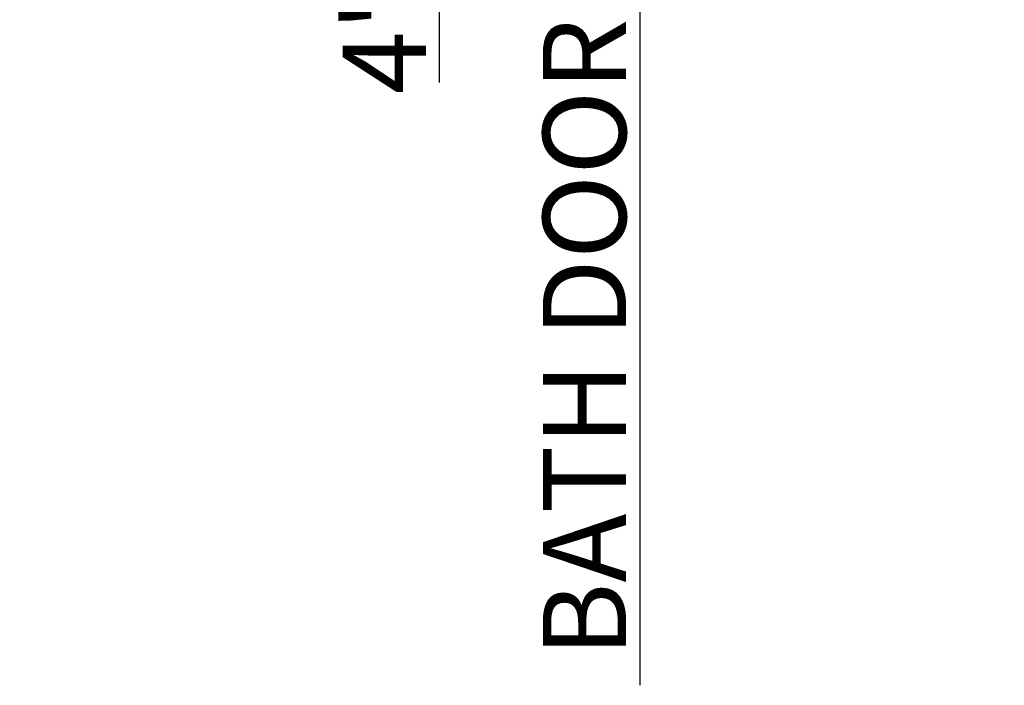
# Model space of a CAD drawing. Units: inches. Extents: x 1102 to 2414, y 295 to 1561.
# Tile 2 of 11: x 1539 to 1965, y 295 to 583. Entities that reach past the tile are written whole.
import ezdxf

# ---------------------------------------------------------------- set-up
doc = ezdxf.new("R2010")
doc.units = ezdxf.units.IN
doc.layers.add('A-ANNO-DIMS', color=2, linetype='Continuous', lineweight=18)
doc.styles.get("Standard").update_dxf_attribs({"font": 'arial.ttf'})
doc.dimstyles.new('ISO-25', dxfattribs={"dimtxt": 36, "dimasz": 24, "dimexe": 1.25, "dimexo": 0.625, "dimtad": 1, "dimlunit": 4, "dimtxsty": 'Standard', "dimcen": 2.5, "dimadec": 0, "dimazin": 0, "dimtfac": 1, "dimtmove": 0, "dimatfit": 3, "dimfxl": 1, "dimarcsym": 0})

# ---------------------------------------------------------------- blocks, each defined once
blk = doc.blocks.new('*D22')
at = {"layer": 'A-ANNO-DIMS', "color": 0, "lineweight": -2, "transparency": 16777216}
for p, q in [((1730.6, 734.42), (1718.75, 734.42)), ((1720, 710.42), (1720, 702.32)), ((1730.6, 678.32), (1718.75, 678.32)), ((1720, 678.32), (1720, 555.92))]:
    blk.add_line(p, q, dxfattribs=at)
at = {"layer": 'A-ANNO-DIMS', "color": 0, "transparency": 16777216}
for points in [[(1716, 710.42), (1724, 710.42), (1720, 734.42)], [(1716, 702.32), (1724, 702.32), (1720, 678.32)]]:
    blk.add_solid(points, dxfattribs=at)
at = {"layer": 'Defpoints', "color": 0, "transparency": 16777216}
for p in [(1731.22, 734.42), (1720, 678.32), (1731.22, 678.32)]:
    blk.add_point(p, dxfattribs=at)
at = {"layer": 'A-ANNO-DIMS', "color": 0, "transparency": 16777216, "insert": (1701, 605.12), "char_height": 36, "attachment_point": 5, "rotation": 90}
blk.add_mtext('4\'-8"', dxfattribs=at)
blk = doc.blocks.new('*D29')
at = {"layer": 'A-ANNO-DIMS', "color": 0, "lineweight": -2, "transparency": 16777216}
for p, q in [((1806.82, 1011.76), (1806.82, 1035.76)), ((1803.17, 987.76), (1808.07, 987.76)), ((1806.82, 987.76), (1806.82, 959.26)), ((1803.17, 959.26), (1808.07, 959.26)), ((1806.82, 935.26), (1806.82, 295.33))]:
    blk.add_line(p, q, dxfattribs=at)
at = {"layer": 'A-ANNO-DIMS', "color": 0, "transparency": 16777216}
for points in [[(1802.82, 1011.76), (1810.82, 1011.76), (1806.82, 987.76)], [(1802.82, 935.26), (1810.82, 935.26), (1806.82, 959.26)]]:
    blk.add_solid(points, dxfattribs=at)
at = {"layer": 'Defpoints', "color": 0, "transparency": 16777216}
for p in [(1802.54, 987.76), (1802.54, 959.26), (1806.82, 959.26)]:
    blk.add_point(p, dxfattribs=at)
at = {"layer": 'A-ANNO-DIMS', "color": 0, "transparency": 16777216, "insert": (1787.57, 603.3), "char_height": 36, "attachment_point": 5, "rotation": 90}
blk.add_mtext('BATH DOOR 2\'-4 1/2" TYP.', dxfattribs=at)
blk = doc.blocks.new('*D42')
at = {"layer": 'A-ANNO-DIMS', "color": 0, "lineweight": -2, "transparency": 16777216}
for p, q in [((1684.54, 645.13), (1684.54, 606.26)), ((1689.04, 645.13), (1689.04, 606.26)), ((1660.54, 607.51), (1636.54, 607.51)), ((1684.54, 607.51), (1689.04, 607.51)), ((1713.04, 607.51), (1917.88, 607.51))]:
    blk.add_line(p, q, dxfattribs=at)
at = {"layer": 'A-ANNO-DIMS', "color": 0, "transparency": 16777216}
for points in [[(1660.54, 611.51), (1660.54, 603.51), (1684.54, 607.51)], [(1713.04, 611.51), (1713.04, 603.51), (1689.04, 607.51)]]:
    blk.add_solid(points, dxfattribs=at)
at = {"layer": 'Defpoints', "color": 0, "transparency": 16777216}
for p in [(1684.54, 645.76), (1689.04, 645.76), (1689.04, 607.51)]:
    blk.add_point(p, dxfattribs=at)
at = {"layer": 'A-ANNO-DIMS', "color": 0, "transparency": 16777216, "insert": (1827.46, 626.75), "char_height": 36, "attachment_point": 5}
blk.add_mtext('0\'-4 1/2"', dxfattribs=at)
blk = doc.blocks.new('*D43')
at = {"layer": 'A-ANNO-DIMS', "color": 0, "lineweight": -2, "transparency": 16777216}
for p, q in [((1586.54, 764.63), (1586.54, 606.26)), ((1629.86, 764.63), (1629.86, 606.26)), ((1562.54, 607.51), (1538.54, 607.51)), ((1586.54, 607.51), (1629.86, 607.51)), ((1653.86, 607.51), (1858.67, 607.51))]:
    blk.add_line(p, q, dxfattribs=at)
at = {"layer": 'A-ANNO-DIMS', "color": 0, "transparency": 16777216}
for points in [[(1562.54, 611.51), (1562.54, 603.51), (1586.54, 607.51)], [(1653.86, 611.51), (1653.86, 603.51), (1629.86, 607.51)]]:
    blk.add_solid(points, dxfattribs=at)
at = {"layer": 'Defpoints', "color": 0, "transparency": 16777216}
for p in [(1586.54, 765.26), (1629.86, 765.26), (1629.86, 607.51)]:
    blk.add_point(p, dxfattribs=at)
at = {"layer": 'A-ANNO-DIMS', "color": 0, "transparency": 16777216, "insert": (1768.27, 626.76), "char_height": 36, "attachment_point": 5}
blk.add_mtext('3\'-7 1/2"', dxfattribs=at)
blk = doc.blocks.new('*D44')
at = {"layer": 'A-ANNO-DIMS', "color": 0, "lineweight": -2, "transparency": 16777216}
for p, q in [((1689.04, 764.63), (1689.04, 606.26)), ((1697.64, 764.63), (1697.64, 606.26)), ((1665.04, 607.51), (1641.04, 607.51)), ((1689.04, 607.51), (1697.64, 607.51)), ((1721.64, 607.51), (1926.48, 607.51))]:
    blk.add_line(p, q, dxfattribs=at)
at = {"layer": 'A-ANNO-DIMS', "color": 0, "transparency": 16777216}
for points in [[(1665.04, 611.51), (1665.04, 603.51), (1689.04, 607.51)], [(1721.64, 611.51), (1721.64, 603.51), (1697.64, 607.51)]]:
    blk.add_solid(points, dxfattribs=at)
at = {"layer": 'Defpoints', "color": 0, "transparency": 16777216}
for p in [(1689.04, 765.26), (1697.64, 765.26), (1697.64, 607.51)]:
    blk.add_point(p, dxfattribs=at)
at = {"layer": 'A-ANNO-DIMS', "color": 0, "transparency": 16777216, "insert": (1836.06, 626.75), "char_height": 36, "attachment_point": 5}
blk.add_mtext('0\'-8 1/2"', dxfattribs=at)
blk = doc.blocks.new('*D46')
at = {"layer": 'A-ANNO-DIMS', "color": 0, "lineweight": -2, "transparency": 16777216}
for p, q in [((1732.04, 857.63), (1732.04, 606.26)), ((1586.54, 853.13), (1586.54, 606.26)), ((1610.54, 607.51), (1708.04, 607.51)), ((1732.04, 607.51), (1961.46, 607.51))]:
    blk.add_line(p, q, dxfattribs=at)
at = {"layer": 'A-ANNO-DIMS', "color": 0, "transparency": 16777216}
for points in [[(1610.54, 611.51), (1610.54, 603.51), (1586.54, 607.51)], [(1708.04, 611.51), (1708.04, 603.51), (1732.04, 607.51)]]:
    blk.add_solid(points, dxfattribs=at)
at = {"layer": 'Defpoints', "color": 0, "transparency": 16777216}
for p in [(1732.04, 858.26), (1586.54, 853.76), (1732.04, 607.51)]:
    blk.add_point(p, dxfattribs=at)
at = {"layer": 'A-ANNO-DIMS', "color": 0, "transparency": 16777216, "insert": (1858.75, 626.75), "char_height": 36, "attachment_point": 5}
blk.add_mtext('12\'-1 1/2"', dxfattribs=at)

msp = doc.modelspace()

# ---------------------------------------------------------------- dimensions: what is measured, and where the dimension line sits
at = {"layer": 'A-ANNO-DIMS'}
dim = msp.add_linear_dim(base=(1806.819, 959.26), p1=(1802.544, 987.76), p2=(1802.544, 959.26), angle=270, text='BATH DOOR <> TYP.', dimstyle='ISO-25', override={"dimdec": 1, "dimlfac": 1, "dimrnd": 0, "dimzin": 1, "dimdsep": 46, "dimlunit": 4, "dimfrac": 2}, dxfattribs=at)
dim.commit()
dim.dimension.update_dxf_attribs({"geometry": '*D29', "text_midpoint": (1787.568, 603.296)})
for base, p1, p2, picture, middle in [((1732.044, 607.51), (1586.544, 853.76), (1732.044, 858.26), '*D46', (1858.751, 626.749)), ((1629.864, 607.51), (1586.544, 765.26), (1629.864, 765.26), '*D43', (1768.268, 626.761)), ((1697.644, 607.51), (1689.044, 765.26), (1697.644, 765.26), '*D44', (1836.06, 626.749)), ((1689.044, 607.51), (1684.544, 645.76), (1689.044, 645.76), '*D42', (1827.46, 626.749))]:
    dim = msp.add_linear_dim(base=base, p1=p1, p2=p2, dimstyle='ISO-25', override={"dimdec": 1, "dimlfac": 1, "dimrnd": 0, "dimzin": 1, "dimdsep": 46, "dimlunit": 4, "dimfrac": 2}, dxfattribs=at)
    dim.commit()
    dim.dimension.update_dxf_attribs({"geometry": picture, "text_midpoint": middle})
dim = msp.add_linear_dim(base=(1720.004, 678.315), p1=(1731.225, 734.418), p2=(1731.225, 678.315), angle=270, dimstyle='ISO-25', override={"dimdec": 1, "dimlfac": 1, "dimrnd": 0, "dimzin": 1, "dimdsep": 46, "dimlunit": 4, "dimfrac": 2}, dxfattribs=at)
dim.commit()
dim.dimension.update_dxf_attribs({"geometry": '*D22', "text_midpoint": (1700.999, 605.118)})

doc.saveas('drawing.dxf')
